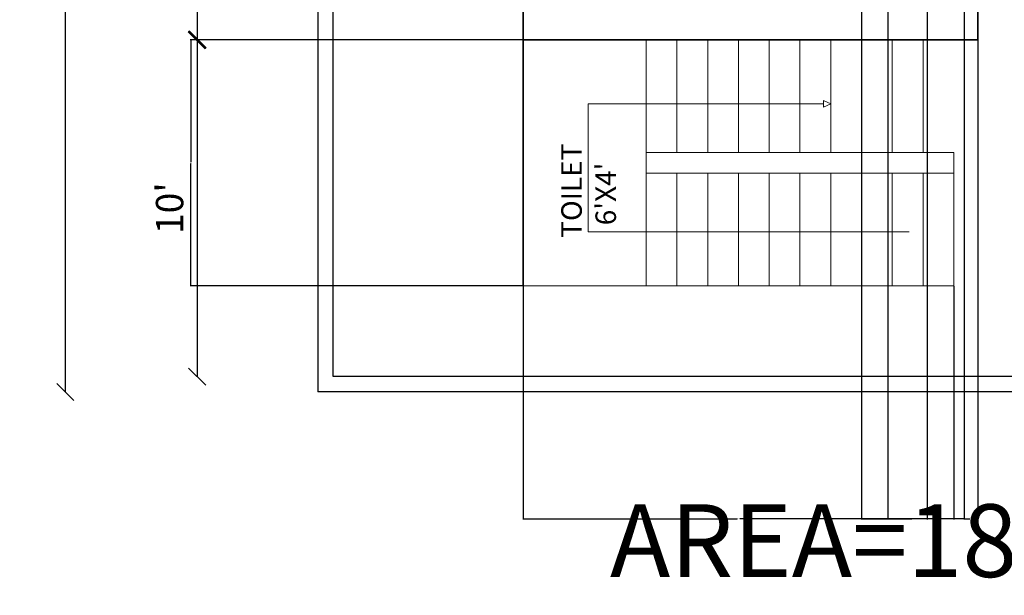
# Model space of a CAD drawing. Units: inches. Extents: x 503 to 1084, y -605 to 132.
# Tile 1 of 14: x 503 to 791, y -605 to -437. Entities that reach past the tile are written whole.
import ezdxf

# ---------------------------------------------------------------- set-up
doc = ezdxf.new("R2010")
doc.units = ezdxf.units.IN
doc.header["$MEASUREMENT"] = 0
for name, color, linetype, lineweight in [('A-ANNO-DIMS', 7, 'Continuous', 18), ('A-ANNO-SYMB', 1, 'Continuous', 13), ('A-ANNO-TEXT', 7, 'Continuous', 18), ('A-AREA-IDEN', 8, 'Continuous', 18), ('A-FLOR-STRS', 1, 'Continuous', 18), ('C-PROP', 1, 'Continuous', 25), ('wall', 1, 'Continuous', 35)]:
    doc.layers.add(name, color=color, linetype=linetype, lineweight=lineweight)
doc.styles.get("Standard").update_dxf_attribs({"font": 'arial.ttf'})
doc.dimstyles.get("Standard").update_dxf_attribs({"dimtxt": 0.18, "dimasz": 0.18, "dimexe": 0.18, "dimexo": 0.0625, "dimgap": 0.09, "dimtad": 0, "dimtih": 1, "dimtoh": 1, "dimdec": 1, "dimzin": 0, "dimdsep": 46, "dimlunit": 4, "dimtxsty": 'Standard', "dimcen": 0.09, "dimadec": 0, "dimazin": 0, "dimtfac": 1, "dimtdec": 1, "dimtofl": 0, "dimtmove": 0, "dimatfit": 3, "dimfxl": 1, "dimtolj": 1, "dimtzin": 0, "dimarcsym": 0})

# ---------------------------------------------------------------- blocks, each defined once
blk = doc.blocks.new('_ArchTick')
at = {"color": 0, "linetype": 'ByBlock', "const_width": 0.15}
blk.add_lwpolyline([(-0.5, -0.5), (0.5, 0.5)], dxfattribs=at)
blk = doc.blocks.new('_Oblique')
at = {"color": 0, "linetype": 'ByBlock', "lineweight": -2}
blk.add_line((-0.5, -0.5), (0.5, 0.5), dxfattribs=at)
blk = doc.blocks.new('*D10')
at = {"layer": 'A-ANNO-DIMS', "color": 0, "lineweight": -2, "transparency": 16777216}
blk.add_line((516.2, 6.18), (516.2, -545.82), dxfattribs=at)
at = {"layer": 'Defpoints', "color": 0, "transparency": 16777216}
for p in [(590.09, 6.18), (516.2, -545.82), (590.09, -545.82)]:
    blk.add_point(p, dxfattribs=at)
at = {"layer": 'A-ANNO-DIMS', "color": 0, "lineweight": -2, "transparency": 16777216, "xscale": 5, "yscale": 5, "zscale": 5}
for name, p, rotation in [('_ArchTick', (516.2, 6.18), 90), ('_Oblique', (516.2, -545.82), 270)]:
    blk.add_blockref(name, p, dxfattribs=dict(at, rotation=rotation))
at = {"layer": 'A-ANNO-DIMS', "color": 0, "transparency": 16777216, "insert": (508.12, -269.82), "char_height": 8, "attachment_point": 5, "rotation": 90}
blk.add_mtext("\\A1;46'", dxfattribs=at)
blk = doc.blocks.new('*D12')
at = {"layer": 'A-ANNO-DIMS', "color": 0, "lineweight": -2, "transparency": 16777216}
blk.add_line((554.79, -17.82), (554.79, -442.82), dxfattribs=at)
at = {"layer": 'Defpoints', "color": 0, "transparency": 16777216}
for p in [(650.09, -17.82), (554.79, -442.82), (650.09, -442.82)]:
    blk.add_point(p, dxfattribs=at)
at = {"layer": 'A-ANNO-DIMS', "color": 0, "lineweight": -2, "transparency": 16777216, "xscale": 5, "yscale": 5, "zscale": 5}
for name, p, rotation in [('_ArchTick', (554.79, -17.82), 90), ('_Oblique', (554.79, -442.82), 270)]:
    blk.add_blockref(name, p, dxfattribs=dict(at, rotation=rotation))
at = {"layer": 'A-ANNO-DIMS', "color": 0, "transparency": 16777216, "insert": (546.7, -230.32), "char_height": 8, "attachment_point": 5, "rotation": 90}
blk.add_mtext("\\A1;36'", dxfattribs=at)
blk = doc.blocks.new('*D13')
at = {"layer": 'A-ANNO-DIMS', "color": 0, "lineweight": -2, "transparency": 16777216}
blk.add_line((554.79, -442.82), (554.79, -541.32), dxfattribs=at)
at = {"layer": 'Defpoints', "color": 0, "transparency": 16777216}
for p in [(650.09, -442.82), (554.79, -541.32), (650.36, -541.32)]:
    blk.add_point(p, dxfattribs=at)
at = {"layer": 'A-ANNO-DIMS', "color": 0, "lineweight": -2, "transparency": 16777216, "xscale": 5, "yscale": 5, "zscale": 5}
for name, p, rotation in [('_ArchTick', (554.79, -442.82), 90), ('_Oblique', (554.79, -541.32), 270)]:
    blk.add_blockref(name, p, dxfattribs=dict(at, rotation=rotation))
at = {"layer": 'A-ANNO-DIMS', "color": 0, "transparency": 16777216, "insert": (546.71, -492.07), "char_height": 8, "attachment_point": 5, "rotation": 90}
blk.add_mtext("\\A1;10'", dxfattribs=at)
blk = doc.blocks.new('*D40')
at = {"layer": 'A-ANNO-DIMS', "color": 0, "lineweight": -2, "transparency": 16777216}
for p, q in [((650.09, -514.88), (650.09, -583.15)), ((776.09, -514.88), (776.09, -583.15)), ((650.27, -582.97), (712.7, -582.97)), ((775.91, -582.97), (713.48, -582.97))]:
    blk.add_line(p, q, dxfattribs=at)
at = {"layer": 'A-ANNO-DIMS', "color": 0, "transparency": 16777216}
for points in [[(650.27, -582.94), (650.27, -583), (650.09, -582.97)], [(775.91, -582.94), (775.91, -583), (776.09, -582.97)]]:
    blk.add_solid(points, dxfattribs=at)
at = {"layer": 'Defpoints', "color": 0, "transparency": 16777216}
for p in [(650.09, -514.82), (776.09, -514.82), (776.09, -582.97)]:
    blk.add_point(p, dxfattribs=at)
at = {"layer": 'A-ANNO-DIMS', "color": 0, "transparency": 16777216, "insert": (713.09, -582.97), "char_height": 0.18, "attachment_point": 5}
blk.add_mtext('\\A1;10\'-6"', dxfattribs=at)
blk = doc.blocks.new('*D41')
at = {"layer": 'A-ANNO-DIMS', "color": 0, "lineweight": -2, "transparency": 16777216}
for p, q in [((650.03, -442.82), (552.76, -442.82)), ((552.94, -443), (552.94, -478.63)), ((552.94, -514.64), (552.94, -479)), ((650.03, -514.82), (552.76, -514.82))]:
    blk.add_line(p, q, dxfattribs=at)
at = {"layer": 'A-ANNO-DIMS', "color": 0, "transparency": 16777216}
for points in [[(552.91, -443), (552.97, -443), (552.94, -442.82)], [(552.91, -514.64), (552.97, -514.64), (552.94, -514.82)]]:
    blk.add_solid(points, dxfattribs=at)
at = {"layer": 'Defpoints', "color": 0, "transparency": 16777216}
for p in [(552.94, -442.82), (650.09, -442.82), (650.09, -514.82)]:
    blk.add_point(p, dxfattribs=at)
at = {"layer": 'A-ANNO-DIMS', "color": 0, "transparency": 16777216, "insert": (552.94, -478.82), "char_height": 0.18, "attachment_point": 5}
blk.add_mtext('\\A1;6\'-0"', dxfattribs=at)
blk = doc.blocks.new('*D60')
at = {"layer": 'A-ANNO-DIMS', "color": 0, "lineweight": -2, "transparency": 16777216}
for p, q in [((749.09, -117.88), (749.09, -583.15)), ((779.09, -117.88), (779.09, -583.15)), ((749.27, -582.97), (763.76, -582.97)), ((778.91, -582.97), (764.42, -582.97))]:
    blk.add_line(p, q, dxfattribs=at)
at = {"layer": 'A-ANNO-DIMS', "color": 0, "transparency": 16777216}
for points in [[(749.27, -582.94), (749.27, -583), (749.09, -582.97)], [(778.91, -582.94), (778.91, -583), (779.09, -582.97)]]:
    blk.add_solid(points, dxfattribs=at)
at = {"layer": 'Defpoints', "color": 0, "transparency": 16777216}
for p in [(749.09, -117.82), (779.09, -117.82), (779.09, -582.97)]:
    blk.add_point(p, dxfattribs=at)
at = {"layer": 'A-ANNO-DIMS', "color": 0, "transparency": 16777216, "insert": (764.09, -582.97), "char_height": 0.18, "attachment_point": 5}
blk.add_mtext('\\A1;2\'-6"', dxfattribs=at)
blk = doc.blocks.new('*D68')
at = {"layer": 'A-ANNO-DIMS', "color": 0, "lineweight": -2, "transparency": 16777216}
for p, q in [((779.09, -117.88), (779.09, -583.15)), ((783.09, -117.88), (783.09, -583.15)), ((779.27, -582.97), (780.76, -582.97)), ((782.91, -582.97), (781.42, -582.97))]:
    blk.add_line(p, q, dxfattribs=at)
at = {"layer": 'A-ANNO-DIMS', "color": 0, "transparency": 16777216}
for points in [[(779.27, -582.94), (779.27, -583), (779.09, -582.97)], [(782.91, -582.94), (782.91, -583), (783.09, -582.97)]]:
    blk.add_solid(points, dxfattribs=at)
at = {"layer": 'Defpoints', "color": 0, "transparency": 16777216}
for p in [(779.09, -117.82), (783.09, -117.82), (783.09, -582.97)]:
    blk.add_point(p, dxfattribs=at)
at = {"layer": 'A-ANNO-DIMS', "color": 0, "transparency": 16777216, "insert": (781.09, -582.97), "char_height": 0.18, "attachment_point": 5}
blk.add_mtext('\\A1;0\'-4"', dxfattribs=at)
blk = doc.blocks.new('*D76')
at = {"layer": 'A-ANNO-DIMS', "color": 0, "lineweight": -2, "transparency": 16777216}
for p, q in [((756.77, -45.47), (756.77, -583.15)), ((768.24, -45.47), (768.24, -583.15)), ((756.95, -582.97), (761.9, -582.97)), ((768.06, -582.97), (763.11, -582.97))]:
    blk.add_line(p, q, dxfattribs=at)
at = {"layer": 'A-ANNO-DIMS', "color": 0, "transparency": 16777216}
for points in [[(756.95, -582.94), (756.95, -583), (756.77, -582.97)], [(768.06, -582.94), (768.06, -583), (768.24, -582.97)]]:
    blk.add_solid(points, dxfattribs=at)
at = {"layer": 'Defpoints', "color": 0, "transparency": 16777216}
for p in [(756.77, -45.4), (768.24, -45.4), (768.24, -582.97)]:
    blk.add_point(p, dxfattribs=at)
at = {"layer": 'A-ANNO-DIMS', "color": 0, "transparency": 16777216, "insert": (762.51, -582.97), "char_height": 0.18, "attachment_point": 5}
blk.add_mtext('\\A1;0\'-11 1/2"', dxfattribs=at)

msp = doc.modelspace()

# ---------------------------------------------------------------- linework, layer by layer
at = {"layer": 'A-ANNO-SYMB'}
for p, q in [((737.95, -461.55), (737.95, -460.55)), ((737.95, -460.55), (740.09, -461.55)), ((669.14, -498.96), (669.14, -461.55)), ((669.14, -461.55), (737.95, -461.55)), ((737.95, -461.55), (737.95, -462.55)), ((737.95, -462.55), (740.09, -461.55)), ((763.07, -498.96), (669.14, -498.96))]:
    msp.add_line(p, q, dxfattribs=at)
at = {"layer": 'A-FLOR-STRS'}
for p, q in [((686.09, -442.82), (686.09, -514.82)), ((695.09, -442.82), (695.09, -475.82)), ((704.09, -442.82), (704.09, -475.82)), ((713.09, -442.82), (713.09, -475.82)), ((722.09, -442.82), (722.09, -475.82)), ((731.09, -442.82), (731.09, -475.82)), ((740.09, -442.82), (740.09, -475.82)), ((749.09, -442.82), (749.09, -475.82)), ((758.09, -442.82), (758.09, -475.82)), ((767.09, -442.82), (767.09, -475.82)), ((686.09, -475.82), (776.09, -475.82)), ((776.09, -475.82), (776.09, -514.82)), ((686.09, -481.82), (776.09, -481.82)), ((695.09, -481.82), (695.09, -514.82)), ((704.09, -481.82), (704.09, -514.82)), ((713.09, -481.82), (713.09, -514.82)), ((722.09, -481.82), (722.09, -514.82)), ((731.09, -481.82), (731.09, -514.82)), ((740.09, -481.82), (740.09, -514.82)), ((749.09, -481.82), (749.09, -514.82)), ((758.09, -481.82), (758.09, -514.82)), ((767.09, -481.82), (767.09, -514.82)), ((650.09, -514.82), (776.09, -514.82))]:
    msp.add_line(p, q, dxfattribs=at)
at = {"layer": 'C-PROP'}
for p, q in [((590.09, 6.18), (590.09, -545.82)), ((594.59, -541.32), (594.59, 1.68)), ((818.09, -541.32), (594.59, -541.32)), ((818.09, -545.82), (590.09, -545.82))]:
    msp.add_line(p, q, dxfattribs=at)
at = {"layer": 'wall'}
for p, q in [((650.09, -17.82), (650.09, -514.82)), ((783.09, -363.82), (783.09, -442.82)), ((650.09, -442.82), (783.09, -442.82))]:
    msp.add_line(p, q, dxfattribs=at)

# ---------------------------------------------------------------- texts
at = {"layer": 'A-ANNO-TEXT', "insert": (675.5, -578.68), "char_height": 21.2807, "attachment_point": 1}
msp.add_mtext_dynamic_manual_height_columns('AREA=1820 SQFT', width=263.9184, gutter_width=3.55, heights=[0], dxfattribs=at)
at = {"layer": 'A-AREA-IDEN', "insert": (661.27, -508.06), "char_height": 6, "attachment_point": 1, "rotation": 90}
msp.add_mtext_dynamic_manual_height_columns("    TOILET\\P      6'X4'", width=54.3765, gutter_width=1, heights=[0], dxfattribs=at)

# ---------------------------------------------------------------- dimensions: what is measured, and where the dimension line sits
at = {"layer": 'A-ANNO-DIMS'}
for base, p1, p2, override, picture, middle in [((516.2, -545.82), (590.09, 6.18), (590.09, -545.82), {"dimtxt": 8, "dimasz": 5, "dimgap": 4, "dimtad": 1, "dimtih": 0, "dimblk1": 'ArchTick', "dimblk2": 'Oblique', "dimsah": 1, "dimse1": 1, "dimse2": 1, "dimclrd": 0, "dimclre": 0, "dimclrt": 0}, '*D10', (508.12, -269.82)), ((552.94, -442.82), (650.09, -514.82), (650.09, -442.82), {"dimdec": 1, "dimlfac": 1, "dimrnd": 0, "dimzin": 1, "dimdsep": 46, "dimlunit": 4, "dimfrac": 2}, '*D41', (552.94, -478.82))]:
    dim = msp.add_linear_dim(base=base, p1=p1, p2=p2, angle=90, dimstyle='Standard', override=override, dxfattribs=at)
    dim.commit()
    dim.dimension.update_dxf_attribs({"geometry": picture, "text_midpoint": middle})
for base, p1, p2, text, picture, middle in [((554.79, -442.82), (650.09, -17.82), (650.09, -442.82), "36'", '*D12', (546.7, -230.32)), ((554.79, -541.32), (650.09, -442.82), (650.36, -541.32), "10'", '*D13', (546.71, -492.07))]:
    dim = msp.add_linear_dim(base=base, p1=p1, p2=p2, angle=90, text=text, dimstyle='Standard', override={"dimtxt": 8, "dimasz": 5, "dimgap": 4, "dimtad": 1, "dimtih": 0, "dimblk1": 'ArchTick', "dimblk2": 'Oblique', "dimsah": 1, "dimse1": 1, "dimse2": 1, "dimclrd": 0, "dimclre": 0, "dimclrt": 0}, dxfattribs=at)
    dim.commit()
    dim.dimension.update_dxf_attribs({"geometry": picture, "text_midpoint": middle})
for base, p1, p2, picture, middle in [((768.24, -582.97), (756.77, -45.4), (768.24, -45.4), '*D76', (762.51, -582.97)), ((779.09, -582.97), (749.09, -117.82), (779.09, -117.82), '*D60', (764.09, -582.97)), ((783.09, -582.97), (779.09, -117.82), (783.09, -117.82), '*D68', (781.09, -582.97)), ((776.09, -582.97), (650.09, -514.82), (776.09, -514.82), '*D40', (713.09, -582.97))]:
    dim = msp.add_linear_dim(base=base, p1=p1, p2=p2, dimstyle='Standard', override={"dimdec": 1, "dimlfac": 1, "dimrnd": 0, "dimzin": 1, "dimdsep": 46, "dimlunit": 4, "dimfrac": 2}, dxfattribs=at)
    dim.commit()
    dim.dimension.update_dxf_attribs({"geometry": picture, "text_midpoint": middle})

doc.saveas('drawing.dxf')
